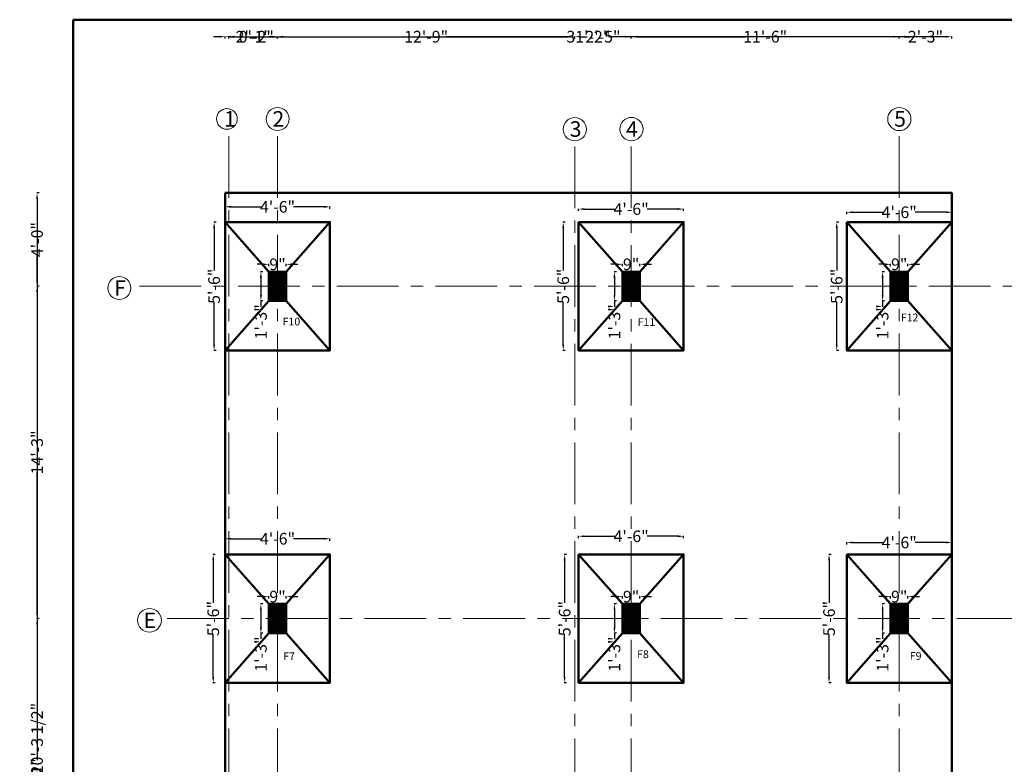
# Model space of a CAD drawing. Units: inches. Extents: x -114 to 953, y -626 to 140.
# Tile 2 of 3: x -114 to 393, y -243 to 140. Entities that reach past the tile are written whole.
import ezdxf

# ---------------------------------------------------------------- set-up
doc = ezdxf.new("R2010")
doc.units = ezdxf.units.IN
doc.header["$MEASUREMENT"] = 0
doc.linetypes.add('CENTER', pattern=[50.8, 31.75, -6.35, 6.35, -6.35])
for name, color, linetype, lineweight in [('S-ANNO-DIMS', 2, 'Continuous', 25), ('S-ANNO-TEXT', 3, 'Continuous', 25), ('S-ANNO-TTLB', 7, 'Continuous', 50), ('S-FNDN', 7, 'Continuous', 50), ('S-GRID', 1, 'CENTER', 18), ('S-GRID-IDEN', 7, 'Continuous', 18)]:
    doc.layers.add(name, color=color, linetype=linetype, lineweight=lineweight)
doc.styles.get("Standard").update_dxf_attribs({"font": 'arial.ttf'})
doc.dimstyles.get("Standard").update_dxf_attribs({"dimtxt": 6, "dimasz": 3, "dimexe": 0.18, "dimexo": 0.0625, "dimgap": 0.09, "dimtad": 0, "dimzin": 0, "dimdsep": 46, "dimlunit": 4, "dimtxsty": 'Standard', "dimcen": 0.09, "dimclrd": 256, "dimclrt": 6, "dimadec": 0, "dimazin": 0, "dimtfac": 6, "dimtofl": 0, "dimtmove": 0, "dimatfit": 3, "dimfxl": 1, "dimfxlon": 1, "dimtolj": 1, "dimtzin": 0, "dimarcsym": 0})

# ---------------------------------------------------------------- blocks, each defined once
blk = doc.blocks.new('*D1')
at = {"layer": 'Defpoints', "color": 0, "transparency": 16777216}
for p in [(14.4, 10.33), (23.4, 14.12), (23.4, 10.33)]:
    blk.add_point(p, dxfattribs=at)
at = {"layer": 'S-ANNO-DIMS', "color": 0, "lineweight": -2, "transparency": 16777216}
for p, q in [((11.4, 14.12), (8.4, 14.12)), ((14.4, 13.12), (14.4, 14.3)), ((23.4, 13.12), (23.4, 14.3)), ((26.4, 14.12), (29.4, 14.12))]:
    blk.add_line(p, q, dxfattribs=at)
at = {"layer": 'S-ANNO-DIMS', "color": 0, "transparency": 16777216}
for points in [[(11.4, 14.62), (11.4, 13.62), (14.4, 14.12)], [(26.4, 14.62), (26.4, 13.62), (23.4, 14.12)]]:
    blk.add_solid(points, dxfattribs=at)
at = {"layer": 'S-ANNO-DIMS', "color": 0, "transparency": 16777216, "insert": (18.9, 14.12), "char_height": 6, "attachment_point": 5}
blk.add_mtext('\\A1;9"', dxfattribs=at)
blk = doc.blocks.new('*D2')
at = {"layer": 'Defpoints', "color": 0, "transparency": 16777216}
for p in [(14.4, 10.33), (10.34, -4.67), (14.4, -4.67)]:
    blk.add_point(p, dxfattribs=at)
at = {"layer": 'S-ANNO-DIMS', "color": 0, "lineweight": -2, "transparency": 16777216}
for p, q in [((11.34, 10.33), (10.16, 10.33)), ((10.34, 7.33), (10.34, -1.67)), ((11.34, -4.67), (10.16, -4.67)), ((10.34, -4.67), (10.34, -7.67))]:
    blk.add_line(p, q, dxfattribs=at)
at = {"layer": 'S-ANNO-DIMS', "color": 0, "transparency": 16777216}
for points in [[(9.84, 7.33), (10.84, 7.33), (10.34, 10.33)], [(9.84, -1.67), (10.84, -1.67), (10.34, -4.67)]]:
    blk.add_solid(points, dxfattribs=at)
at = {"layer": 'S-ANNO-DIMS', "color": 0, "transparency": 16777216, "insert": (10.34, -15.45), "char_height": 6, "attachment_point": 5, "rotation": 90}
blk.add_mtext('\\A1;1\'-3"', dxfattribs=at)
blk = doc.blocks.new('*D3')
at = {"layer": 'Defpoints', "color": 0, "transparency": 16777216}
for p in [(334.4, 10.33), (343.4, 14.12), (343.4, 10.33)]:
    blk.add_point(p, dxfattribs=at)
at = {"layer": 'S-ANNO-DIMS', "color": 0, "lineweight": -2, "transparency": 16777216}
for p, q in [((331.4, 14.12), (328.4, 14.12)), ((334.4, 13.12), (334.4, 14.3)), ((343.4, 13.12), (343.4, 14.3)), ((346.4, 14.12), (349.4, 14.12))]:
    blk.add_line(p, q, dxfattribs=at)
at = {"layer": 'S-ANNO-DIMS', "color": 0, "transparency": 16777216}
for points in [[(331.4, 14.62), (331.4, 13.62), (334.4, 14.12)], [(346.4, 14.62), (346.4, 13.62), (343.4, 14.12)]]:
    blk.add_solid(points, dxfattribs=at)
at = {"layer": 'S-ANNO-DIMS', "color": 0, "transparency": 16777216, "insert": (338.9, 14.12), "char_height": 6, "attachment_point": 5}
blk.add_mtext('\\A1;9"', dxfattribs=at)
blk = doc.blocks.new('*D4')
at = {"layer": 'Defpoints', "color": 0, "transparency": 16777216}
for p in [(334.4, 10.33), (330.34, -4.67), (334.4, -4.67)]:
    blk.add_point(p, dxfattribs=at)
at = {"layer": 'S-ANNO-DIMS', "color": 0, "lineweight": -2, "transparency": 16777216}
for p, q in [((331.34, 10.33), (330.16, 10.33)), ((330.34, 7.33), (330.34, -1.67)), ((331.34, -4.67), (330.16, -4.67)), ((330.34, -4.67), (330.34, -7.67))]:
    blk.add_line(p, q, dxfattribs=at)
at = {"layer": 'S-ANNO-DIMS', "color": 0, "transparency": 16777216}
for points in [[(329.84, 7.33), (330.84, 7.33), (330.34, 10.33)], [(329.84, -1.67), (330.84, -1.67), (330.34, -4.67)]]:
    blk.add_solid(points, dxfattribs=at)
at = {"layer": 'S-ANNO-DIMS', "color": 0, "transparency": 16777216, "insert": (330.34, -15.45), "char_height": 6, "attachment_point": 5, "rotation": 90}
blk.add_mtext('\\A1;1\'-3"', dxfattribs=at)
blk = doc.blocks.new('*D5')
at = {"layer": 'Defpoints', "color": 0, "transparency": 16777216}
for p in [(23.4, -156.88), (14.4, -160.67), (23.4, -160.67)]:
    blk.add_point(p, dxfattribs=at)
at = {"layer": 'S-ANNO-DIMS', "color": 0, "lineweight": -2, "transparency": 16777216}
for p, q in [((11.4, -156.88), (8.4, -156.88)), ((14.4, -157.88), (14.4, -156.7)), ((23.4, -157.88), (23.4, -156.7)), ((26.4, -156.88), (29.4, -156.88))]:
    blk.add_line(p, q, dxfattribs=at)
at = {"layer": 'S-ANNO-DIMS', "color": 0, "transparency": 16777216}
for points in [[(11.4, -156.38), (11.4, -157.38), (14.4, -156.88)], [(26.4, -156.38), (26.4, -157.38), (23.4, -156.88)]]:
    blk.add_solid(points, dxfattribs=at)
at = {"layer": 'S-ANNO-DIMS', "color": 0, "transparency": 16777216, "insert": (18.9, -156.88), "char_height": 6, "attachment_point": 5}
blk.add_mtext('\\A1;9"', dxfattribs=at)
blk = doc.blocks.new('*D6')
at = {"layer": 'Defpoints', "color": 0, "transparency": 16777216}
for p in [(14.4, -160.67), (10.34, -175.67), (14.4, -175.67)]:
    blk.add_point(p, dxfattribs=at)
at = {"layer": 'S-ANNO-DIMS', "color": 0, "lineweight": -2, "transparency": 16777216}
for p, q in [((11.34, -160.67), (10.16, -160.67)), ((10.34, -163.67), (10.34, -172.67)), ((11.34, -175.67), (10.16, -175.67)), ((10.34, -175.67), (10.34, -178.67))]:
    blk.add_line(p, q, dxfattribs=at)
at = {"layer": 'S-ANNO-DIMS', "color": 0, "transparency": 16777216}
for points in [[(9.84, -163.67), (10.84, -163.67), (10.34, -160.67)], [(9.84, -172.67), (10.84, -172.67), (10.34, -175.67)]]:
    blk.add_solid(points, dxfattribs=at)
at = {"layer": 'S-ANNO-DIMS', "color": 0, "transparency": 16777216, "insert": (10.34, -186.45), "char_height": 6, "attachment_point": 5, "rotation": 90}
blk.add_mtext('\\A1;1\'-3"', dxfattribs=at)
blk = doc.blocks.new('*D7')
at = {"layer": 'Defpoints', "color": 0, "transparency": 16777216}
for p in [(343.4, -156.88), (334.4, -160.67), (343.4, -160.67)]:
    blk.add_point(p, dxfattribs=at)
at = {"layer": 'S-ANNO-DIMS', "color": 0, "lineweight": -2, "transparency": 16777216}
for p, q in [((331.4, -156.88), (328.4, -156.88)), ((334.4, -157.88), (334.4, -156.7)), ((343.4, -157.88), (343.4, -156.7)), ((346.4, -156.88), (349.4, -156.88))]:
    blk.add_line(p, q, dxfattribs=at)
at = {"layer": 'S-ANNO-DIMS', "color": 0, "transparency": 16777216}
for points in [[(331.4, -156.38), (331.4, -157.38), (334.4, -156.88)], [(346.4, -156.38), (346.4, -157.38), (343.4, -156.88)]]:
    blk.add_solid(points, dxfattribs=at)
at = {"layer": 'S-ANNO-DIMS', "color": 0, "transparency": 16777216, "insert": (338.9, -156.88), "char_height": 6, "attachment_point": 5}
blk.add_mtext('\\A1;9"', dxfattribs=at)
blk = doc.blocks.new('*D8')
at = {"layer": 'Defpoints', "color": 0, "transparency": 16777216}
for p in [(334.4, -160.67), (330.34, -175.67), (334.4, -175.67)]:
    blk.add_point(p, dxfattribs=at)
at = {"layer": 'S-ANNO-DIMS', "color": 0, "lineweight": -2, "transparency": 16777216}
for p, q in [((331.34, -160.67), (330.16, -160.67)), ((330.34, -163.67), (330.34, -172.67)), ((331.34, -175.67), (330.16, -175.67)), ((330.34, -175.67), (330.34, -178.67))]:
    blk.add_line(p, q, dxfattribs=at)
at = {"layer": 'S-ANNO-DIMS', "color": 0, "transparency": 16777216}
for points in [[(329.84, -163.67), (330.84, -163.67), (330.34, -160.67)], [(329.84, -172.67), (330.84, -172.67), (330.34, -175.67)]]:
    blk.add_solid(points, dxfattribs=at)
at = {"layer": 'S-ANNO-DIMS', "color": 0, "transparency": 16777216, "insert": (330.34, -186.45), "char_height": 6, "attachment_point": 5, "rotation": 90}
blk.add_mtext('\\A1;1\'-3"', dxfattribs=at)
blk = doc.blocks.new('*D15')
at = {"layer": 'Defpoints', "color": 0, "transparency": 16777216}
for p in [(196.4, 10.33), (205.4, 14.12), (205.4, 10.33)]:
    blk.add_point(p, dxfattribs=at)
at = {"layer": 'S-ANNO-DIMS', "color": 0, "lineweight": -2, "transparency": 16777216}
for p, q in [((193.4, 14.12), (190.4, 14.12)), ((196.4, 13.12), (196.4, 14.3)), ((205.4, 13.12), (205.4, 14.3)), ((208.4, 14.12), (211.4, 14.12))]:
    blk.add_line(p, q, dxfattribs=at)
at = {"layer": 'S-ANNO-DIMS', "color": 0, "transparency": 16777216}
for points in [[(193.4, 14.62), (193.4, 13.62), (196.4, 14.12)], [(208.4, 14.62), (208.4, 13.62), (205.4, 14.12)]]:
    blk.add_solid(points, dxfattribs=at)
at = {"layer": 'S-ANNO-DIMS', "color": 0, "transparency": 16777216, "insert": (200.9, 14.12), "char_height": 6, "attachment_point": 5}
blk.add_mtext('\\A1;9"', dxfattribs=at)
blk = doc.blocks.new('*D16')
at = {"layer": 'Defpoints', "color": 0, "transparency": 16777216}
for p in [(196.4, 10.33), (192.33, -4.67), (196.4, -4.67)]:
    blk.add_point(p, dxfattribs=at)
at = {"layer": 'S-ANNO-DIMS', "color": 0, "lineweight": -2, "transparency": 16777216}
for p, q in [((193.33, 10.33), (192.15, 10.33)), ((192.33, 7.33), (192.33, -1.67)), ((193.33, -4.67), (192.15, -4.67)), ((192.33, -4.67), (192.33, -7.67))]:
    blk.add_line(p, q, dxfattribs=at)
at = {"layer": 'S-ANNO-DIMS', "color": 0, "transparency": 16777216}
for points in [[(191.83, 7.33), (192.83, 7.33), (192.33, 10.33)], [(191.83, -1.67), (192.83, -1.67), (192.33, -4.67)]]:
    blk.add_solid(points, dxfattribs=at)
at = {"layer": 'S-ANNO-DIMS', "color": 0, "transparency": 16777216, "insert": (192.33, -15.45), "char_height": 6, "attachment_point": 5, "rotation": 90}
blk.add_mtext('\\A1;1\'-3"', dxfattribs=at)
blk = doc.blocks.new('*D17')
at = {"layer": 'Defpoints', "color": 0, "transparency": 16777216}
for p in [(205.4, -156.88), (196.4, -160.67), (205.4, -160.67)]:
    blk.add_point(p, dxfattribs=at)
at = {"layer": 'S-ANNO-DIMS', "color": 0, "lineweight": -2, "transparency": 16777216}
for p, q in [((193.4, -156.88), (190.4, -156.88)), ((196.4, -157.88), (196.4, -156.7)), ((205.4, -157.88), (205.4, -156.7)), ((208.4, -156.88), (211.4, -156.88))]:
    blk.add_line(p, q, dxfattribs=at)
at = {"layer": 'S-ANNO-DIMS', "color": 0, "transparency": 16777216}
for points in [[(193.4, -156.38), (193.4, -157.38), (196.4, -156.88)], [(208.4, -156.38), (208.4, -157.38), (205.4, -156.88)]]:
    blk.add_solid(points, dxfattribs=at)
at = {"layer": 'S-ANNO-DIMS', "color": 0, "transparency": 16777216, "insert": (200.9, -156.88), "char_height": 6, "attachment_point": 5}
blk.add_mtext('\\A1;9"', dxfattribs=at)
blk = doc.blocks.new('*D18')
at = {"layer": 'Defpoints', "color": 0, "transparency": 16777216}
for p in [(196.4, -160.67), (192.33, -175.67), (196.4, -175.67)]:
    blk.add_point(p, dxfattribs=at)
at = {"layer": 'S-ANNO-DIMS', "color": 0, "lineweight": -2, "transparency": 16777216}
for p, q in [((193.33, -160.67), (192.15, -160.67)), ((192.33, -163.67), (192.33, -172.67)), ((193.33, -175.67), (192.15, -175.67)), ((192.33, -175.67), (192.33, -178.67))]:
    blk.add_line(p, q, dxfattribs=at)
at = {"layer": 'S-ANNO-DIMS', "color": 0, "transparency": 16777216}
for points in [[(191.83, -163.67), (192.83, -163.67), (192.33, -160.67)], [(191.83, -172.67), (192.83, -172.67), (192.33, -175.67)]]:
    blk.add_solid(points, dxfattribs=at)
at = {"layer": 'S-ANNO-DIMS', "color": 0, "transparency": 16777216, "insert": (192.33, -186.45), "char_height": 6, "attachment_point": 5, "rotation": 90}
blk.add_mtext('\\A1;1\'-3"', dxfattribs=at)
blk = doc.blocks.new('*D21')
at = {"layer": 'Defpoints', "color": 0, "transparency": 16777216}
for p in [(45.9, 43.7), (-8.1, 35.83), (45.9, 35.83)]:
    blk.add_point(p, dxfattribs=at)
at = {"layer": 'S-ANNO-DIMS', "color": 0, "lineweight": -2, "transparency": 16777216}
for p, q in [((-8.1, 42.7), (-8.1, 43.88)), ((-5.1, 43.7), (10.72, 43.7)), ((42.9, 43.7), (27.09, 43.7)), ((45.9, 42.7), (45.9, 43.88))]:
    blk.add_line(p, q, dxfattribs=at)
at = {"layer": 'S-ANNO-DIMS', "color": 0, "transparency": 16777216}
for points in [[(-5.1, 44.2), (-5.1, 43.2), (-8.1, 43.7)], [(42.9, 44.2), (42.9, 43.2), (45.9, 43.7)]]:
    blk.add_solid(points, dxfattribs=at)
at = {"layer": 'S-ANNO-DIMS', "color": 0, "transparency": 16777216, "insert": (18.9, 43.7), "char_height": 6, "attachment_point": 5}
blk.add_mtext('\\A1;4\'-6"', dxfattribs=at)
blk = doc.blocks.new('*D22')
at = {"layer": 'Defpoints', "color": 0, "transparency": 16777216}
for p in [(-8.1, 35.83), (-13.75, -30.17), (-8.1, -30.17)]:
    blk.add_point(p, dxfattribs=at)
at = {"layer": 'S-ANNO-DIMS', "color": 0, "lineweight": -2, "transparency": 16777216}
for p, q in [((-12.75, 35.83), (-13.93, 35.83)), ((-13.75, 32.83), (-13.75, 10.9)), ((-13.75, -27.17), (-13.75, -5.23)), ((-12.75, -30.17), (-13.93, -30.17))]:
    blk.add_line(p, q, dxfattribs=at)
at = {"layer": 'S-ANNO-DIMS', "color": 0, "transparency": 16777216}
for points in [[(-14.25, 32.83), (-13.25, 32.83), (-13.75, 35.83)], [(-14.25, -27.17), (-13.25, -27.17), (-13.75, -30.17)]]:
    blk.add_solid(points, dxfattribs=at)
at = {"layer": 'S-ANNO-DIMS', "color": 0, "transparency": 16777216, "insert": (-13.75, 2.83), "char_height": 6, "attachment_point": 5, "rotation": 90}
blk.add_mtext('\\A1;5\'-6"', dxfattribs=at)
blk = doc.blocks.new('*D23')
at = {"layer": 'Defpoints', "color": 0, "transparency": 16777216}
for p in [(227.9, 42.57), (173.9, 35.83), (227.9, 35.83)]:
    blk.add_point(p, dxfattribs=at)
at = {"layer": 'S-ANNO-DIMS', "color": 0, "lineweight": -2, "transparency": 16777216}
for p, q in [((173.9, 41.57), (173.9, 42.75)), ((176.9, 42.57), (192.71, 42.57)), ((224.9, 42.57), (209.08, 42.57)), ((227.9, 41.57), (227.9, 42.75))]:
    blk.add_line(p, q, dxfattribs=at)
at = {"layer": 'S-ANNO-DIMS', "color": 0, "transparency": 16777216}
for points in [[(176.9, 43.07), (176.9, 42.07), (173.9, 42.57)], [(224.9, 43.07), (224.9, 42.07), (227.9, 42.57)]]:
    blk.add_solid(points, dxfattribs=at)
at = {"layer": 'S-ANNO-DIMS', "color": 0, "transparency": 16777216, "insert": (200.9, 42.57), "char_height": 6, "attachment_point": 5}
blk.add_mtext('\\A1;4\'-6"', dxfattribs=at)
blk = doc.blocks.new('*D24')
at = {"layer": 'Defpoints', "color": 0, "transparency": 16777216}
for p in [(173.9, 35.83), (165.96, -30.17), (173.9, -30.17)]:
    blk.add_point(p, dxfattribs=at)
at = {"layer": 'S-ANNO-DIMS', "color": 0, "lineweight": -2, "transparency": 16777216}
for p, q in [((166.96, 35.83), (165.78, 35.83)), ((165.96, 32.83), (165.96, 10.9)), ((165.96, -27.17), (165.96, -5.23)), ((166.96, -30.17), (165.78, -30.17))]:
    blk.add_line(p, q, dxfattribs=at)
at = {"layer": 'S-ANNO-DIMS', "color": 0, "transparency": 16777216}
for points in [[(165.46, 32.83), (166.46, 32.83), (165.96, 35.83)], [(165.46, -27.17), (166.46, -27.17), (165.96, -30.17)]]:
    blk.add_solid(points, dxfattribs=at)
at = {"layer": 'S-ANNO-DIMS', "color": 0, "transparency": 16777216, "insert": (165.96, 2.83), "char_height": 6, "attachment_point": 5, "rotation": 90}
blk.add_mtext('\\A1;5\'-6"', dxfattribs=at)
blk = doc.blocks.new('*D25')
at = {"layer": 'Defpoints', "color": 0, "transparency": 16777216}
for p in [(365.9, 40.92), (311.9, 35.83), (365.9, 35.83)]:
    blk.add_point(p, dxfattribs=at)
at = {"layer": 'S-ANNO-DIMS', "color": 0, "lineweight": -2, "transparency": 16777216}
for p, q in [((311.9, 39.92), (311.9, 41.1)), ((314.9, 40.92), (330.72, 40.92)), ((362.9, 40.92), (347.09, 40.92)), ((365.9, 39.92), (365.9, 41.1))]:
    blk.add_line(p, q, dxfattribs=at)
at = {"layer": 'S-ANNO-DIMS', "color": 0, "transparency": 16777216}
for points in [[(314.9, 41.42), (314.9, 40.42), (311.9, 40.92)], [(362.9, 41.42), (362.9, 40.42), (365.9, 40.92)]]:
    blk.add_solid(points, dxfattribs=at)
at = {"layer": 'S-ANNO-DIMS', "color": 0, "transparency": 16777216, "insert": (338.9, 40.92), "char_height": 6, "attachment_point": 5}
blk.add_mtext('\\A1;4\'-6"', dxfattribs=at)
blk = doc.blocks.new('*D26')
at = {"layer": 'Defpoints', "color": 0, "transparency": 16777216}
for p in [(311.9, 35.83), (306.74, -30.17), (311.9, -30.17)]:
    blk.add_point(p, dxfattribs=at)
at = {"layer": 'S-ANNO-DIMS', "color": 0, "lineweight": -2, "transparency": 16777216}
for p, q in [((307.74, 35.83), (306.56, 35.83)), ((306.74, 32.83), (306.74, 10.9)), ((306.74, -27.17), (306.74, -5.23)), ((307.74, -30.17), (306.56, -30.17))]:
    blk.add_line(p, q, dxfattribs=at)
at = {"layer": 'S-ANNO-DIMS', "color": 0, "transparency": 16777216}
for points in [[(306.24, 32.83), (307.24, 32.83), (306.74, 35.83)], [(306.24, -27.17), (307.24, -27.17), (306.74, -30.17)]]:
    blk.add_solid(points, dxfattribs=at)
at = {"layer": 'S-ANNO-DIMS', "color": 0, "transparency": 16777216, "insert": (306.74, 2.83), "char_height": 6, "attachment_point": 5, "rotation": 90}
blk.add_mtext('\\A1;5\'-6"', dxfattribs=at)
blk = doc.blocks.new('*D27')
at = {"layer": 'Defpoints', "color": 0, "transparency": 16777216}
for p in [(45.9, -127.1), (-8.1, -135.17), (45.9, -135.17)]:
    blk.add_point(p, dxfattribs=at)
at = {"layer": 'S-ANNO-DIMS', "color": 0, "lineweight": -2, "transparency": 16777216}
for p, q in [((-8.1, -128.1), (-8.1, -126.92)), ((-5.1, -127.1), (10.72, -127.1)), ((42.9, -127.1), (27.09, -127.1)), ((45.9, -128.1), (45.9, -126.92))]:
    blk.add_line(p, q, dxfattribs=at)
at = {"layer": 'S-ANNO-DIMS', "color": 0, "transparency": 16777216}
for points in [[(-5.1, -126.6), (-5.1, -127.6), (-8.1, -127.1)], [(42.9, -126.6), (42.9, -127.6), (45.9, -127.1)]]:
    blk.add_solid(points, dxfattribs=at)
at = {"layer": 'S-ANNO-DIMS', "color": 0, "transparency": 16777216, "insert": (18.9, -127.1), "char_height": 6, "attachment_point": 5}
blk.add_mtext('\\A1;4\'-6"', dxfattribs=at)
blk = doc.blocks.new('*D28')
at = {"layer": 'Defpoints', "color": 0, "transparency": 16777216}
for p in [(-8.1, -135.17), (-14.21, -201.17), (-8.1, -201.17)]:
    blk.add_point(p, dxfattribs=at)
at = {"layer": 'S-ANNO-DIMS', "color": 0, "lineweight": -2, "transparency": 16777216}
for p, q in [((-13.21, -135.17), (-14.39, -135.17)), ((-14.21, -138.17), (-14.21, -160.1)), ((-14.21, -198.17), (-14.21, -176.23)), ((-13.21, -201.17), (-14.39, -201.17))]:
    blk.add_line(p, q, dxfattribs=at)
at = {"layer": 'S-ANNO-DIMS', "color": 0, "transparency": 16777216}
for points in [[(-14.71, -138.17), (-13.71, -138.17), (-14.21, -135.17)], [(-14.71, -198.17), (-13.71, -198.17), (-14.21, -201.17)]]:
    blk.add_solid(points, dxfattribs=at)
at = {"layer": 'S-ANNO-DIMS', "color": 0, "transparency": 16777216, "insert": (-14.21, -168.17), "char_height": 6, "attachment_point": 5, "rotation": 90}
blk.add_mtext('\\A1;5\'-6"', dxfattribs=at)
blk = doc.blocks.new('*D29')
at = {"layer": 'Defpoints', "color": 0, "transparency": 16777216}
for p in [(227.9, -125.83), (173.9, -135.17), (227.9, -135.17)]:
    blk.add_point(p, dxfattribs=at)
at = {"layer": 'S-ANNO-DIMS', "color": 0, "lineweight": -2, "transparency": 16777216}
for p, q in [((173.9, -126.83), (173.9, -125.65)), ((176.9, -125.83), (192.71, -125.83)), ((224.9, -125.83), (209.08, -125.83)), ((227.9, -126.83), (227.9, -125.65))]:
    blk.add_line(p, q, dxfattribs=at)
at = {"layer": 'S-ANNO-DIMS', "color": 0, "transparency": 16777216}
for points in [[(176.9, -125.33), (176.9, -126.33), (173.9, -125.83)], [(224.9, -125.33), (224.9, -126.33), (227.9, -125.83)]]:
    blk.add_solid(points, dxfattribs=at)
at = {"layer": 'S-ANNO-DIMS', "color": 0, "transparency": 16777216, "insert": (200.9, -125.83), "char_height": 6, "attachment_point": 5}
blk.add_mtext('\\A1;4\'-6"', dxfattribs=at)
blk = doc.blocks.new('*D30')
at = {"layer": 'Defpoints', "color": 0, "transparency": 16777216}
for p in [(173.9, -135.17), (166.68, -201.17), (173.9, -201.17)]:
    blk.add_point(p, dxfattribs=at)
at = {"layer": 'S-ANNO-DIMS', "color": 0, "lineweight": -2, "transparency": 16777216}
for p, q in [((167.68, -135.17), (166.5, -135.17)), ((166.68, -138.17), (166.68, -160.1)), ((166.68, -198.17), (166.68, -176.23)), ((167.68, -201.17), (166.5, -201.17))]:
    blk.add_line(p, q, dxfattribs=at)
at = {"layer": 'S-ANNO-DIMS', "color": 0, "transparency": 16777216}
for points in [[(166.18, -138.17), (167.18, -138.17), (166.68, -135.17)], [(166.18, -198.17), (167.18, -198.17), (166.68, -201.17)]]:
    blk.add_solid(points, dxfattribs=at)
at = {"layer": 'S-ANNO-DIMS', "color": 0, "transparency": 16777216, "insert": (166.68, -168.17), "char_height": 6, "attachment_point": 5, "rotation": 90}
blk.add_mtext('\\A1;5\'-6"', dxfattribs=at)
blk = doc.blocks.new('*D31')
at = {"layer": 'Defpoints', "color": 0, "transparency": 16777216}
for p in [(365.9, -129.04), (311.9, -135.17), (365.9, -135.17)]:
    blk.add_point(p, dxfattribs=at)
at = {"layer": 'S-ANNO-DIMS', "color": 0, "lineweight": -2, "transparency": 16777216}
for p, q in [((311.9, -130.04), (311.9, -128.86)), ((314.9, -129.04), (330.72, -129.04)), ((362.9, -129.04), (347.09, -129.04)), ((365.9, -130.04), (365.9, -128.86))]:
    blk.add_line(p, q, dxfattribs=at)
at = {"layer": 'S-ANNO-DIMS', "color": 0, "transparency": 16777216}
for points in [[(314.9, -128.54), (314.9, -129.54), (311.9, -129.04)], [(362.9, -128.54), (362.9, -129.54), (365.9, -129.04)]]:
    blk.add_solid(points, dxfattribs=at)
at = {"layer": 'S-ANNO-DIMS', "color": 0, "transparency": 16777216, "insert": (338.9, -129.04), "char_height": 6, "attachment_point": 5}
blk.add_mtext('\\A1;4\'-6"', dxfattribs=at)
blk = doc.blocks.new('*D32')
at = {"layer": 'Defpoints', "color": 0, "transparency": 16777216}
for p in [(311.9, -135.17), (302.79, -201.17), (311.9, -201.17)]:
    blk.add_point(p, dxfattribs=at)
at = {"layer": 'S-ANNO-DIMS', "color": 0, "lineweight": -2, "transparency": 16777216}
for p, q in [((303.79, -135.17), (302.61, -135.17)), ((302.79, -138.17), (302.79, -160.1)), ((302.79, -198.17), (302.79, -176.23)), ((303.79, -201.17), (302.61, -201.17))]:
    blk.add_line(p, q, dxfattribs=at)
at = {"layer": 'S-ANNO-DIMS', "color": 0, "transparency": 16777216}
for points in [[(302.29, -138.17), (303.29, -138.17), (302.79, -135.17)], [(302.29, -198.17), (303.29, -198.17), (302.79, -201.17)]]:
    blk.add_solid(points, dxfattribs=at)
at = {"layer": 'S-ANNO-DIMS', "color": 0, "transparency": 16777216, "insert": (302.79, -168.17), "char_height": 6, "attachment_point": 5, "rotation": 90}
blk.add_mtext('\\A1;5\'-6"', dxfattribs=at)
blk = doc.blocks.new('FOOTING-ISOL-COL')
h = blk.add_hatch()
h.set_pattern_fill('2X2µØ×©', color=256)
h.set_pattern_definition([(0, (379.9615, 68.9256), (0.5, 0.5), [0.45, -0.05, 0.2, -0.05, 0.2, -0.05]), (0, (379.9615, 69.1256), (0.5, 0.5), [0.45, -0.55]), (0, (379.9615, 69.1756), (0.5, 0.5), [0.45, -0.55]), (0, (379.9615, 69.3756), (0.5, 0.5), [0.45, -0.05, 0.2, -0.05, 0.2, -0.05]), (90, (379.9615, 68.9256), (-0.5, 0.5), [0.2, -0.05, 0.2, -0.05, 0.45, -0.05]), (90, (380.4115, 68.9256), (-0.5, 0.5), [0.2, -0.05, 0.2, -0.05, 0.45, -0.05]), (90, (380.6615, 68.9256), (-0.5, 0.5), [0.45, -0.55]), (90, (380.7115, 68.9256), (-0.5, 0.5), [0.45, -0.55])])
h.paths.add_polyline_path([(23.4, 10.33), (14.4, 10.33), (14.4, -4.67), (23.4, -4.67)])
for p, q in [((14.4, 10.33), (-8.1, 35.83)), ((23.4, 10.33), (45.9, 35.83)), ((14.4, -4.67), (-8.1, -30.17)), ((23.4, -4.67), (45.9, -30.17))]:
    blk.add_line(p, q)
for points in [[(-8.1, 35.83), (45.9, 35.83), (45.9, -30.17), (-8.1, -30.17)], [(14.4, 10.33), (23.4, 10.33), (23.4, -4.67), (14.4, -4.67)]]:
    blk.add_lwpolyline(points, close=True)
blk = doc.blocks.new('*D49')
at = {"layer": 'Defpoints', "color": 0, "transparency": 16777216}
for p in [(18.9, 131.26), (-6.1, 80.05), (18.9, 80.05)]:
    blk.add_point(p, dxfattribs=at)
at = {"layer": 'S-ANNO-DIMS', "color": 0, "lineweight": -2, "transparency": 16777216}
for p, q in [((-6.1, 130.26), (-6.1, 131.44)), ((18.9, 130.26), (18.9, 131.44))]:
    blk.add_line(p, q, dxfattribs=at)
at = {"layer": 'S-ANNO-DIMS', "lineweight": -2, "transparency": 16777216}
for p, q in [((-3.1, 131.26), (-1.71, 131.26)), ((15.9, 131.26), (14.52, 131.26))]:
    blk.add_line(p, q, dxfattribs=at)
at = {"layer": 'S-ANNO-DIMS', "transparency": 16777216}
for points in [[(-3.1, 131.76), (-3.1, 130.76), (-6.1, 131.26)], [(15.9, 131.76), (15.9, 130.76), (18.9, 131.26)]]:
    blk.add_solid(points, dxfattribs=at)
at = {"layer": 'S-ANNO-DIMS', "color": 6, "transparency": 16777216, "insert": (6.4, 131.26), "char_height": 6, "attachment_point": 5}
blk.add_mtext('\\A1;2\'-1"', dxfattribs=at)
blk = doc.blocks.new('*D50')
at = {"layer": 'Defpoints', "color": 0, "transparency": 16777216}
for p in [(171.9, 131.26), (18.9, 80.05), (171.9, 74.83)]:
    blk.add_point(p, dxfattribs=at)
at = {"layer": 'S-ANNO-DIMS', "color": 0, "lineweight": -2, "transparency": 16777216}
for p, q in [((18.9, 130.26), (18.9, 131.44)), ((171.9, 130.26), (171.9, 131.44))]:
    blk.add_line(p, q, dxfattribs=at)
at = {"layer": 'S-ANNO-DIMS', "lineweight": -2, "transparency": 16777216}
for p, q in [((21.9, 131.26), (85.29, 131.26)), ((168.9, 131.26), (105.51, 131.26))]:
    blk.add_line(p, q, dxfattribs=at)
at = {"layer": 'S-ANNO-DIMS', "transparency": 16777216}
for points in [[(21.9, 131.76), (21.9, 130.76), (18.9, 131.26)], [(168.9, 131.76), (168.9, 130.76), (171.9, 131.26)]]:
    blk.add_solid(points, dxfattribs=at)
at = {"layer": 'S-ANNO-DIMS', "color": 6, "transparency": 16777216, "insert": (95.4, 131.26), "char_height": 6, "attachment_point": 5}
blk.add_mtext('\\A1;12\'-9"', dxfattribs=at)
blk = doc.blocks.new('*D51')
at = {"layer": 'Defpoints', "color": 0, "transparency": 16777216}
for p in [(200.9, 131.26), (171.9, 74.83), (200.9, 74.83)]:
    blk.add_point(p, dxfattribs=at)
at = {"layer": 'S-ANNO-DIMS', "color": 0, "lineweight": -2, "transparency": 16777216}
for p, q in [((171.9, 130.26), (171.9, 131.44)), ((200.9, 130.26), (200.9, 131.44))]:
    blk.add_line(p, q, dxfattribs=at)
at = {"layer": 'S-ANNO-DIMS', "lineweight": -2, "transparency": 16777216}
for p, q in [((174.9, 131.26), (178.28, 131.26)), ((197.9, 131.26), (194.51, 131.26))]:
    blk.add_line(p, q, dxfattribs=at)
at = {"layer": 'S-ANNO-DIMS', "transparency": 16777216}
for points in [[(174.9, 131.76), (174.9, 130.76), (171.9, 131.26)], [(197.9, 131.76), (197.9, 130.76), (200.9, 131.26)]]:
    blk.add_solid(points, dxfattribs=at)
at = {"layer": 'S-ANNO-DIMS', "color": 6, "transparency": 16777216, "insert": (186.4, 131.26), "char_height": 6, "attachment_point": 5}
blk.add_mtext('\\A1;2\'-5"', dxfattribs=at)
blk = doc.blocks.new('*D52')
at = {"layer": 'Defpoints', "color": 0, "transparency": 16777216}
for p in [(338.9, 131.26), (338.9, 80.05), (200.9, 74.83)]:
    blk.add_point(p, dxfattribs=at)
at = {"layer": 'S-ANNO-DIMS', "color": 0, "lineweight": -2, "transparency": 16777216}
for p, q in [((200.9, 130.26), (200.9, 131.44)), ((338.9, 130.26), (338.9, 131.44))]:
    blk.add_line(p, q, dxfattribs=at)
at = {"layer": 'S-ANNO-DIMS', "lineweight": -2, "transparency": 16777216}
for p, q in [((203.9, 131.26), (259.79, 131.26)), ((335.9, 131.26), (280.01, 131.26))]:
    blk.add_line(p, q, dxfattribs=at)
at = {"layer": 'S-ANNO-DIMS', "transparency": 16777216}
for points in [[(203.9, 131.76), (203.9, 130.76), (200.9, 131.26)], [(335.9, 131.76), (335.9, 130.76), (338.9, 131.26)]]:
    blk.add_solid(points, dxfattribs=at)
at = {"layer": 'S-ANNO-DIMS', "color": 6, "transparency": 16777216, "insert": (269.9, 131.26), "char_height": 6, "attachment_point": 5}
blk.add_mtext('\\A1;11\'-6"', dxfattribs=at)
blk = doc.blocks.new('*D53')
at = {"layer": 'Defpoints', "color": 0, "transparency": 16777216}
for p in [(365.9, 131.26), (-8.1, 50.84), (365.9, 50.84)]:
    blk.add_point(p, dxfattribs=at)
at = {"layer": 'S-ANNO-DIMS', "color": 0, "lineweight": -2, "transparency": 16777216}
for p, q in [((-8.1, 130.26), (-8.1, 131.44)), ((365.9, 130.26), (365.9, 131.44))]:
    blk.add_line(p, q, dxfattribs=at)
at = {"layer": 'S-ANNO-DIMS', "lineweight": -2, "transparency": 16777216}
for p, q in [((-5.1, 131.26), (168.51, 131.26)), ((362.9, 131.26), (189.3, 131.26))]:
    blk.add_line(p, q, dxfattribs=at)
at = {"layer": 'S-ANNO-DIMS', "transparency": 16777216}
for points in [[(-5.1, 131.76), (-5.1, 130.76), (-8.1, 131.26)], [(362.9, 131.76), (362.9, 130.76), (365.9, 131.26)]]:
    blk.add_solid(points, dxfattribs=at)
at = {"layer": 'S-ANNO-DIMS', "color": 6, "transparency": 16777216, "insert": (178.9, 131.26), "char_height": 6, "attachment_point": 5}
blk.add_mtext('\\A1;31\'-2"', dxfattribs=at)
blk = doc.blocks.new('*D54')
at = {"layer": 'Defpoints', "color": 0, "transparency": 16777216}
for p in [(-6.1, 131.26), (-6.1, 80.05), (-8.1, 50.84)]:
    blk.add_point(p, dxfattribs=at)
at = {"layer": 'S-ANNO-DIMS', "lineweight": -2, "transparency": 16777216}
for p, q in [((-11.1, 131.26), (-14.1, 131.26)), ((-3.1, 131.26), (-0.1, 131.26))]:
    blk.add_line(p, q, dxfattribs=at)
at = {"layer": 'S-ANNO-DIMS', "color": 0, "lineweight": -2, "transparency": 16777216}
for p, q in [((-8.1, 130.26), (-8.1, 131.44)), ((-6.1, 130.26), (-6.1, 131.44))]:
    blk.add_line(p, q, dxfattribs=at)
at = {"layer": 'S-ANNO-DIMS', "transparency": 16777216}
for points in [[(-11.1, 131.76), (-11.1, 130.76), (-8.1, 131.26)], [(-3.1, 131.76), (-3.1, 130.76), (-6.1, 131.26)]]:
    blk.add_solid(points, dxfattribs=at)
at = {"layer": 'S-ANNO-DIMS', "color": 6, "transparency": 16777216, "insert": (7.97, 131.26), "char_height": 6, "attachment_point": 5}
blk.add_mtext('\\A1;0\'-2"', dxfattribs=at)
blk = doc.blocks.new('*D55')
at = {"layer": 'Defpoints', "color": 0, "transparency": 16777216}
for p in [(365.9, 131.26), (338.9, 80.05), (365.9, 50.84)]:
    blk.add_point(p, dxfattribs=at)
at = {"layer": 'S-ANNO-DIMS', "color": 0, "lineweight": -2, "transparency": 16777216}
for p, q in [((338.9, 130.26), (338.9, 131.44)), ((365.9, 130.26), (365.9, 131.44))]:
    blk.add_line(p, q, dxfattribs=at)
at = {"layer": 'S-ANNO-DIMS', "lineweight": -2, "transparency": 16777216}
for p, q in [((341.9, 131.26), (344.29, 131.26)), ((362.9, 131.26), (360.52, 131.26))]:
    blk.add_line(p, q, dxfattribs=at)
at = {"layer": 'S-ANNO-DIMS', "transparency": 16777216}
for points in [[(341.9, 131.76), (341.9, 130.76), (338.9, 131.26)], [(362.9, 131.76), (362.9, 130.76), (365.9, 131.26)]]:
    blk.add_solid(points, dxfattribs=at)
at = {"layer": 'S-ANNO-DIMS', "color": 6, "transparency": 16777216, "insert": (352.4, 131.26), "char_height": 6, "attachment_point": 5}
blk.add_mtext('\\A1;2\'-3"', dxfattribs=at)
blk = doc.blocks.new('*D56')
at = {"layer": 'Defpoints', "color": 0, "transparency": 16777216}
for p in [(-52.22, 2.83), (-104.87, -168.17), (-37.87, -168.17)]:
    blk.add_point(p, dxfattribs=at)
at = {"layer": 'S-ANNO-DIMS', "color": 0, "lineweight": -2, "transparency": 16777216}
for p, q in [((-103.87, 2.83), (-105.05, 2.83)), ((-103.87, -168.17), (-105.05, -168.17))]:
    blk.add_line(p, q, dxfattribs=at)
at = {"layer": 'S-ANNO-DIMS', "lineweight": -2, "transparency": 16777216}
for p, q in [((-104.87, -0.17), (-104.87, -72.56)), ((-104.87, -165.17), (-104.87, -92.78))]:
    blk.add_line(p, q, dxfattribs=at)
at = {"layer": 'S-ANNO-DIMS', "transparency": 16777216}
for points in [[(-105.37, -0.17), (-104.37, -0.17), (-104.87, 2.83)], [(-105.37, -165.17), (-104.37, -165.17), (-104.87, -168.17)]]:
    blk.add_solid(points, dxfattribs=at)
at = {"layer": 'S-ANNO-DIMS', "color": 6, "transparency": 16777216, "insert": (-104.87, -82.67), "char_height": 6, "attachment_point": 5, "rotation": 90}
blk.add_mtext('\\A1;14\'-3"', dxfattribs=at)
blk = doc.blocks.new('*D57')
at = {"layer": 'Defpoints', "color": 0, "transparency": 16777216}
for p in [(-37.87, -168.17), (-104.87, -291.67), (-37.87, -291.67)]:
    blk.add_point(p, dxfattribs=at)
at = {"layer": 'S-ANNO-DIMS', "color": 0, "lineweight": -2, "transparency": 16777216}
for p, q in [((-103.87, -168.17), (-105.05, -168.17)), ((-103.87, -291.67), (-105.05, -291.67))]:
    blk.add_line(p, q, dxfattribs=at)
at = {"layer": 'S-ANNO-DIMS', "lineweight": -2, "transparency": 16777216}
for p, q in [((-104.87, -171.17), (-104.87, -212.81)), ((-104.87, -288.67), (-104.87, -247.02))]:
    blk.add_line(p, q, dxfattribs=at)
at = {"layer": 'S-ANNO-DIMS', "transparency": 16777216}
for points in [[(-105.37, -171.17), (-104.37, -171.17), (-104.87, -168.17)], [(-105.37, -288.67), (-104.37, -288.67), (-104.87, -291.67)]]:
    blk.add_solid(points, dxfattribs=at)
at = {"layer": 'S-ANNO-DIMS', "color": 6, "transparency": 16777216, "insert": (-104.87, -229.92), "char_height": 6, "attachment_point": 5, "rotation": 90}
blk.add_mtext('\\A1;10\'-3 1/2"', dxfattribs=at)
blk = doc.blocks.new('*D61')
at = {"layer": 'Defpoints', "color": 0, "transparency": 16777216}
for p in [(-8.1, 50.84), (-104.87, 2.83), (-52.22, 2.83)]:
    blk.add_point(p, dxfattribs=at)
at = {"layer": 'S-ANNO-DIMS', "color": 0, "lineweight": -2, "transparency": 16777216}
for p, q in [((-103.87, 50.84), (-105.05, 50.84)), ((-103.87, 2.83), (-105.05, 2.83))]:
    blk.add_line(p, q, dxfattribs=at)
at = {"layer": 'S-ANNO-DIMS', "lineweight": -2, "transparency": 16777216}
for p, q in [((-104.87, 47.84), (-104.87, 35.02)), ((-104.87, 5.83), (-104.87, 18.65))]:
    blk.add_line(p, q, dxfattribs=at)
at = {"layer": 'S-ANNO-DIMS', "transparency": 16777216}
for points in [[(-105.37, 47.84), (-104.37, 47.84), (-104.87, 50.84)], [(-105.37, 5.83), (-104.37, 5.83), (-104.87, 2.83)]]:
    blk.add_solid(points, dxfattribs=at)
at = {"layer": 'S-ANNO-DIMS', "color": 6, "transparency": 16777216, "insert": (-104.87, 26.84), "char_height": 6, "attachment_point": 5, "rotation": 90}
blk.add_mtext('\\A1;4\'-0"', dxfattribs=at)
blk = doc.blocks.new('*D63')
at = {"layer": 'Defpoints', "color": 0, "transparency": 16777216}
for p in [(-8.1, 50.84), (-104.87, -567.67), (-8.1, -567.67)]:
    blk.add_point(p, dxfattribs=at)
at = {"layer": 'S-ANNO-DIMS', "color": 0, "lineweight": -2, "transparency": 16777216}
for p, q in [((-103.87, 50.84), (-105.05, 50.84)), ((-103.87, -567.67), (-105.05, -567.67))]:
    blk.add_line(p, q, dxfattribs=at)
at = {"layer": 'S-ANNO-DIMS', "lineweight": -2, "transparency": 16777216}
for p, q in [((-104.87, 47.84), (-104.87, -241.03)), ((-104.87, -564.67), (-104.87, -275.8))]:
    blk.add_line(p, q, dxfattribs=at)
at = {"layer": 'S-ANNO-DIMS', "transparency": 16777216}
for points in [[(-105.37, 47.84), (-104.37, 47.84), (-104.87, 50.84)], [(-105.37, -564.67), (-104.37, -564.67), (-104.87, -567.67)]]:
    blk.add_solid(points, dxfattribs=at)
at = {"layer": 'S-ANNO-DIMS', "color": 6, "transparency": 16777216, "insert": (-104.87, -258.41), "char_height": 6, "attachment_point": 5, "rotation": 90}
blk.add_mtext('\\A1;51\'-6 1/2"', dxfattribs=at)

msp = doc.modelspace()

# ---------------------------------------------------------------- linework, layer by layer
at = {"layer": 'S-ANNO-TTLB'}
msp.add_lwpolyline([(-86.343, 140.009), (953.065, 140.009), (953.065, -626.35), (-86.343, -626.35)], close=True, dxfattribs=at)
at = {"layer": 'S-FNDN'}
msp.add_lwpolyline([(-8.098, 50.843), (365.902, 50.843), (365.902, -567.669), (-8.098, -567.669)], close=True, dxfattribs=at)
at = {"layer": 'S-GRID'}
for p, q in [((-6.098, 80.047), (-6.098, -534.669)), ((18.902, 80.047), (18.902, -626.35)), ((338.902, 80.047), (338.902, -626.35)), ((171.897, 74.831), (171.897, -626.35)), ((200.897, 74.831), (200.897, -626.35)), ((-52.223, 2.831), (403.662, 2.831)), ((-37.867, -168.169), (403.662, -168.169))]:
    msp.add_line(p, q, dxfattribs=at)
at = {"layer": 'S-GRID-IDEN'}
for centre, radius in [((-7.17, 88.934), 5.326), ((18.953, 88.934), 5.924), ((338.955, 88.882), 5.968), ((171.918, 83.647), 5.965), ((201.066, 83.735), 5.98), ((-62.53, 1.931), 5.94), ((-47.013, -169.069), 6.113)]:
    msp.add_circle(centre, radius, dxfattribs=at)

# ---------------------------------------------------------------- block references
at = {"layer": 'S-FNDN'}
for p in [(0, 0), (181.996, 0), (320, 0), (0, -171), (181.996, -171), (320, -171)]:
    msp.add_blockref('FOOTING-ISOL-COL', p, dxfattribs=at)

# ---------------------------------------------------------------- texts
at = {"layer": 'S-ANNO-TEXT', "char_height": 4, "attachment_point": 1}
for s, insert in [('{\\fArial|b1|i0|c0|p34;F10}', (21.502, -13.339)), ('{\\fArial|b1|i0|c0|p34;F11}', (204.26, -13.59)), ('{\\fArial|b1|i0|c0|p34;F12}', (339.712, -11.219)), ('{\\fArial|b1|i0|c0|p34;F7}', (21.817, -185.571)), ('{\\fArial|b1|i0|c0|p34;F8}', (203.981, -184.524)), ('{\\fArial|b1|i0|c0|p34;F9}', (344.34, -185.395))]:
    msp.add_mtext_dynamic_manual_height_columns(s, width=16.75606, gutter_width=1, heights=[0], dxfattribs=dict(at, insert=insert))
at = {"layer": 'S-GRID-IDEN', "char_height": 8, "attachment_point": 1}
for s, insert in [('1', (-8.644, 92.95)), ('2', (16.303, 92.95)), ('5', (336.303, 92.95)), ('3', (169.299, 87.735)), ('4', (198.299, 87.735)), ('F', (-65.229, 5.931)), ('E', (-49.998, -165.069))]:
    msp.add_mtext_dynamic_manual_height_columns(s, width=16.75606, gutter_width=1, heights=[0], dxfattribs=dict(at, insert=insert))

# ---------------------------------------------------------------- dimensions: what is measured, and where the dimension line sits
at = {"layer": 'S-ANNO-DIMS'}
for base, p1, p2, override, picture, middle in [((-6.098, 131.258), (-8.098, 50.843), (-6.098, 80.047), {"dimdec": 1, "dimlfac": 1, "dimrnd": 0, "dimzin": 1, "dimdsep": 46, "dimlunit": 4, "dimfrac": 2}, '*D54', (7.966, 131.258)), ((365.902, 131.258), (-8.098, 50.843), (365.902, 50.843), {"dimdec": 1, "dimlfac": 1, "dimrnd": 0, "dimzin": 1, "dimdsep": 46, "dimlunit": 4, "dimfrac": 2}, '*D53', (178.902, 131.258)), ((18.902, 131.258), (-6.098, 80.047), (18.902, 80.047), {"dimdec": 1, "dimlfac": 1, "dimrnd": 0, "dimzin": 1, "dimdsep": 46, "dimlunit": 4, "dimfrac": 2}, '*D49', (6.402, 131.258)), ((171.897, 131.258), (18.902, 80.047), (171.897, 74.831), {"dimdec": 1, "dimlfac": 1, "dimrnd": 0, "dimzin": 1, "dimdsep": 46, "dimlunit": 4, "dimfrac": 2}, '*D50', (95.399, 131.258)), ((200.897, 131.258), (171.897, 74.831), (200.897, 74.831), {"dimdec": 1, "dimlfac": 1, "dimrnd": 0, "dimzin": 1, "dimdsep": 46, "dimlunit": 4, "dimfrac": 2}, '*D51', (186.397, 131.258)), ((338.902, 131.258), (200.897, 74.831), (338.902, 80.047), {"dimdec": 1, "dimlfac": 1, "dimrnd": 0, "dimzin": 1, "dimdsep": 46, "dimlunit": 4, "dimfrac": 2}, '*D52', (269.899, 131.258)), ((365.902, 131.258), (338.902, 80.047), (365.902, 50.843), {"dimdec": 1, "dimlfac": 1, "dimrnd": 0, "dimzin": 1, "dimdsep": 46, "dimlunit": 4, "dimfrac": 2}, '*D55', (352.402, 131.258)), ((45.902, 43.705), (-8.098, 35.831), (45.902, 35.831), {"dimclrd": 0, "dimclre": 0, "dimclrt": 0}, '*D21', (18.902, 43.705)), ((227.897, 42.574), (173.897, 35.831), (227.897, 35.831), {"dimclrd": 0, "dimclre": 0, "dimclrt": 0}, '*D23', (200.897, 42.574)), ((365.902, 40.922), (311.902, 35.831), (365.902, 35.831), {"dimclrd": 0, "dimclre": 0, "dimclrt": 0}, '*D25', (338.902, 40.922)), ((23.402, 14.125), (14.402, 10.331), (23.402, 10.331), {"dimclrd": 0, "dimclre": 0, "dimclrt": 0}, '*D1', (18.902, 14.125)), ((205.397, 14.125), (196.397, 10.331), (205.397, 10.331), {"dimclrd": 0, "dimclre": 0, "dimclrt": 0}, '*D15', (200.897, 14.125)), ((343.402, 14.125), (334.402, 10.331), (343.402, 10.331), {"dimclrd": 0, "dimclre": 0, "dimclrt": 0}, '*D3', (338.902, 14.125)), ((45.902, -127.101), (-8.098, -135.169), (45.902, -135.169), {"dimclrd": 0, "dimclre": 0, "dimclrt": 0}, '*D27', (18.902, -127.101)), ((227.897, -125.828), (173.897, -135.169), (227.897, -135.169), {"dimclrd": 0, "dimclre": 0, "dimclrt": 0}, '*D29', (200.897, -125.828)), ((365.902, -129.039), (311.902, -135.169), (365.902, -135.169), {"dimclrd": 0, "dimclre": 0, "dimclrt": 0}, '*D31', (338.902, -129.039)), ((23.402, -156.875), (14.402, -160.669), (23.402, -160.669), {"dimclrd": 0, "dimclre": 0, "dimclrt": 0}, '*D5', (18.902, -156.875)), ((205.397, -156.875), (196.397, -160.669), (205.397, -160.669), {"dimclrd": 0, "dimclre": 0, "dimclrt": 0}, '*D17', (200.897, -156.875)), ((343.402, -156.875), (334.402, -160.669), (343.402, -160.669), {"dimclrd": 0, "dimclre": 0, "dimclrt": 0}, '*D7', (338.902, -156.875))]:
    dim = msp.add_linear_dim(base=base, p1=p1, p2=p2, dimstyle='Standard', override=override, dxfattribs=at)
    dim.commit()
    dim.dimension.update_dxf_attribs({"geometry": picture, "text_midpoint": middle})
for base, p1, p2, override, picture, middle in [((-104.87, -567.669), (-8.098, 50.843), (-8.098, -567.669), {"dimdec": 1, "dimlfac": 1, "dimrnd": 0, "dimzin": 1, "dimdsep": 46, "dimlunit": 4, "dimfrac": 2}, '*D63', (-104.87, -258.413)), ((-104.87, 2.831), (-8.098, 50.843), (-52.223, 2.831), {"dimdec": 1, "dimlfac": 1, "dimrnd": 0, "dimzin": 1, "dimdsep": 46, "dimlunit": 4, "dimfrac": 2}, '*D61', (-104.87, 26.837)), ((-13.754, -30.169), (-8.098, 35.831), (-8.098, -30.169), {"dimclrd": 0, "dimclre": 0, "dimclrt": 0}, '*D22', (-13.754, 2.831)), ((165.958, -30.169), (173.897, 35.831), (173.897, -30.169), {"dimclrd": 0, "dimclre": 0, "dimclrt": 0}, '*D24', (165.958, 2.831)), ((306.743, -30.169), (311.902, 35.831), (311.902, -30.169), {"dimclrd": 0, "dimclre": 0, "dimclrt": 0}, '*D26', (306.743, 2.831)), ((10.338, -4.669), (14.402, 10.331), (14.402, -4.669), {"dimclrd": 0, "dimclre": 0, "dimclrt": 0}, '*D2', (10.338, -15.451)), ((192.334, -4.669), (196.397, 10.331), (196.397, -4.669), {"dimclrd": 0, "dimclre": 0, "dimclrt": 0}, '*D16', (192.334, -15.451)), ((330.338, -4.669), (334.402, 10.331), (334.402, -4.669), {"dimclrd": 0, "dimclre": 0, "dimclrt": 0}, '*D4', (330.338, -15.451)), ((-104.87, -168.169), (-52.223, 2.831), (-37.867, -168.169), {"dimdec": 1, "dimlfac": 1, "dimrnd": 0, "dimzin": 1, "dimdsep": 46, "dimlunit": 4, "dimfrac": 2}, '*D56', (-104.87, -82.669)), ((-14.214, -201.169), (-8.098, -135.169), (-8.098, -201.169), {"dimclrd": 0, "dimclre": 0, "dimclrt": 0}, '*D28', (-14.214, -168.169)), ((166.681, -201.169), (173.897, -135.169), (173.897, -201.169), {"dimclrd": 0, "dimclre": 0, "dimclrt": 0}, '*D30', (166.681, -168.169)), ((302.793, -201.169), (311.902, -135.169), (311.902, -201.169), {"dimclrd": 0, "dimclre": 0, "dimclrt": 0}, '*D32', (302.793, -168.169)), ((10.338, -175.669), (14.402, -160.669), (14.402, -175.669), {"dimclrd": 0, "dimclre": 0, "dimclrt": 0}, '*D6', (10.338, -186.451)), ((192.334, -175.669), (196.397, -160.669), (196.397, -175.669), {"dimclrd": 0, "dimclre": 0, "dimclrt": 0}, '*D18', (192.334, -186.451)), ((330.338, -175.669), (334.402, -160.669), (334.402, -175.669), {"dimclrd": 0, "dimclre": 0, "dimclrt": 0}, '*D8', (330.338, -186.451)), ((-104.87, -291.669), (-37.867, -168.169), (-37.867, -291.669), {"dimdec": 1, "dimlfac": 1, "dimrnd": 0, "dimzin": 1, "dimdsep": 46, "dimlunit": 4, "dimfrac": 2}, '*D57', (-104.87, -229.919))]:
    dim = msp.add_linear_dim(base=base, p1=p1, p2=p2, angle=90, dimstyle='Standard', override=override, dxfattribs=at)
    dim.commit()
    dim.dimension.update_dxf_attribs({"geometry": picture, "text_midpoint": middle})

doc.saveas('drawing.dxf')
